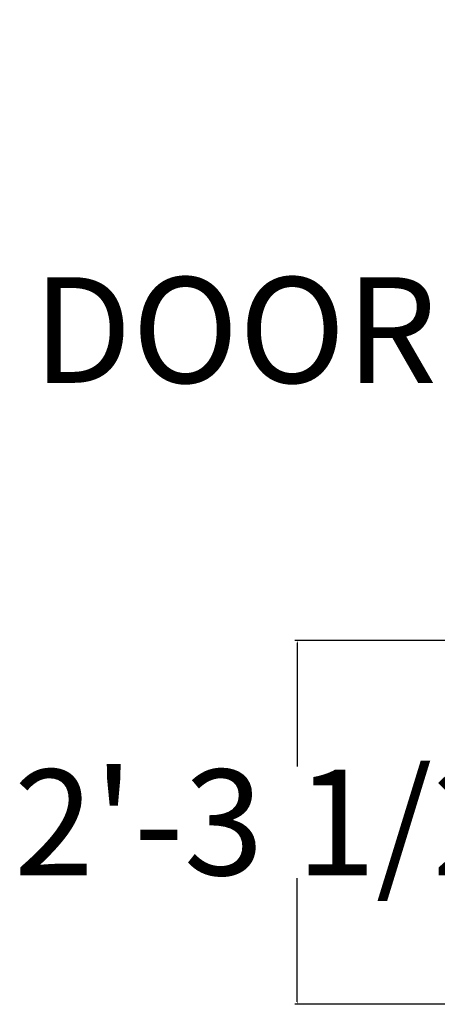
# Model space of a CAD drawing. Units: inches. Extents: x 638 to 1303, y 1 to 699.
# Tile 12 of 21: x 995 to 1026, y 412 to 487. Entities that reach past the tile are written whole.
import ezdxf

# ---------------------------------------------------------------- set-up
doc = ezdxf.new("R2010")
doc.units = ezdxf.units.IN
doc.header["$MEASUREMENT"] = 0
doc.layers.add('A-ANNO-DIMS', color=2, linetype='Continuous', lineweight=18)
doc.styles.get("Standard").update_dxf_attribs({"font": 'arial.ttf'})
doc.dimstyles.get("Standard").update_dxf_attribs({"dimtxt": 8, "dimasz": 0.18, "dimexe": 0.18, "dimexo": 0.0625, "dimgap": 0.09, "dimtad": 0, "dimtih": 1, "dimtoh": 1, "dimdec": 4, "dimzin": 0, "dimdsep": 46, "dimlunit": 3, "dimtxsty": 'Standard', "dimcen": 0.09, "dimadec": 0, "dimazin": 0, "dimtfac": 1, "dimtdec": 4, "dimtofl": 0, "dimtmove": 0, "dimatfit": 3, "dimfxl": 1, "dimtolj": 1, "dimtzin": 0, "dimarcsym": 0})

# ---------------------------------------------------------------- blocks, each defined once
blk = doc.blocks.new('*D26')
at = {"layer": 'A-ANNO-DIMS', "color": 0, "lineweight": -2, "transparency": 16777216}
for p, q in [((1046.675, 486.875), (1039.508, 486.875)), ((1039.688, 486.695), (1039.688, 467.606)), ((1039.688, 440.055), (1039.688, 459.143)), ((1046.675, 439.875), (1039.508, 439.875))]:
    blk.add_line(p, q, dxfattribs=at)
at = {"layer": 'A-ANNO-DIMS', "color": 0, "transparency": 16777216}
for points in [[(1039.658, 486.695), (1039.718, 486.695), (1039.688, 486.875)], [(1039.658, 440.055), (1039.718, 440.055), (1039.688, 439.875)]]:
    blk.add_solid(points, dxfattribs=at)
at = {"layer": 'Defpoints', "color": 0, "transparency": 16777216}
for p in [(1046.738, 486.875), (1039.688, 439.875), (1046.738, 439.875)]:
    blk.add_point(p, dxfattribs=at)
at = {"layer": 'A-ANNO-DIMS', "color": 0, "transparency": 16777216, "insert": (1039.688, 463.375), "char_height": 8, "attachment_point": 5}
blk.add_mtext('\\A1;DOOR 3\'-11" TYP.', dxfattribs=at)
blk = doc.blocks.new('*D65')
at = {"layer": 'A-ANNO-DIMS', "color": 0, "lineweight": -2, "transparency": 16777216}
for p, q in [((1051.175, 439.875), (1015.558, 439.875)), ((1015.738, 439.695), (1015.738, 430.326)), ((1015.738, 412.499), (1015.738, 421.868)), ((1051.175, 412.319), (1015.558, 412.319))]:
    blk.add_line(p, q, dxfattribs=at)
at = {"layer": 'A-ANNO-DIMS', "color": 0, "transparency": 16777216}
for points in [[(1015.708, 439.695), (1015.768, 439.695), (1015.738, 439.875)], [(1015.708, 412.499), (1015.768, 412.499), (1015.738, 412.319)]]:
    blk.add_solid(points, dxfattribs=at)
at = {"layer": 'Defpoints', "color": 0, "transparency": 16777216}
for p in [(1015.738, 439.875), (1051.238, 439.875), (1051.238, 412.319)]:
    blk.add_point(p, dxfattribs=at)
at = {"layer": 'A-ANNO-DIMS', "color": 0, "transparency": 16777216, "insert": (1015.738, 426.097), "char_height": 8, "attachment_point": 5}
blk.add_mtext('\\A1;2\'-3 1/2"', dxfattribs=at)

msp = doc.modelspace()

# ---------------------------------------------------------------- dimensions: what is measured, and where the dimension line sits
at = {"layer": 'A-ANNO-DIMS'}
dim = msp.add_linear_dim(base=(1039.68798, 439.87457), p1=(1046.73798, 486.87457), p2=(1046.73798, 439.87457), angle=270, text='DOOR <> TYP.', dimstyle='Standard', override={"dimdec": 1, "dimlfac": 1, "dimrnd": 0, "dimzin": 1, "dimdsep": 46, "dimlunit": 4, "dimfrac": 2}, dxfattribs=at)
dim.commit()
dim.dimension.update_dxf_attribs({"geometry": '*D26', "text_midpoint": (1039.68798, 463.37457)})
dim = msp.add_linear_dim(base=(1015.73798, 439.87457), p1=(1051.23798, 412.31895), p2=(1051.23798, 439.87457), angle=90, dimstyle='Standard', override={"dimdec": 1, "dimlfac": 1, "dimrnd": 0, "dimzin": 1, "dimdsep": 46, "dimlunit": 4, "dimfrac": 2}, dxfattribs=at)
dim.commit()
dim.dimension.update_dxf_attribs({"geometry": '*D65', "text_midpoint": (1015.73798, 426.09676)})

doc.saveas('drawing.dxf')
